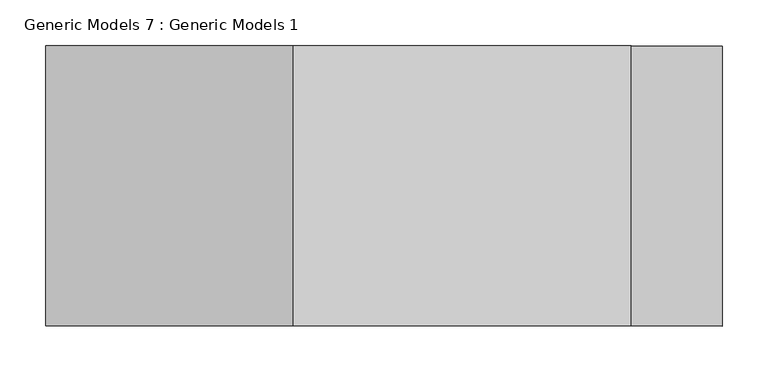
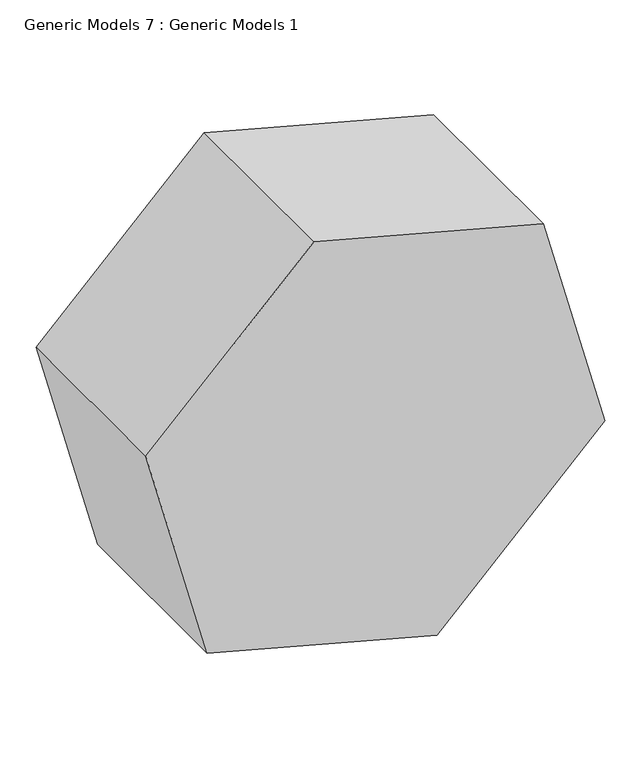
"""IFC4 building model written with IfcOpenShell, lengths in millimetres: proxy geometry, Generic Models 7 : Generic Models 1."""

from ifc_helpers import new_model, si_unit, frame, origin, place, context, project, spatial, polyline, outline, extrude, source, transform, mapped, element, save


def generic_models_7_generic_models_1_35c4f0a6(model_context):
    return source(origin(), model_context, "Body", "SweptSolid", [
        extrude(outline(polyline([(904.7566299, -4463.0070438), (1003.366686, -4831.0247836), (733.9590024, -5100.4324672), (365.9412626, -5001.822411), (267.3312064, -4633.8046712), (536.73889, -4364.3969876), (904.7566299, -4463.0070438)])), frame((0.0, -9086.6225464, 0.0), z_axis=(0.0, 1.0, 0.0), x_axis=(0.0, 0.0, 1.0)), (0.0, 0.0, 1.0), 304.8),
    ])


if __name__ == "__main__":
    model = new_model("IFC4")
    model_context = context("Model", 3, world=origin())
    ifc_project = project(units=[si_unit("LENGTHUNIT", "METRE", prefix="MILLI")], contexts=[model_context])
    site = spatial("IfcSite", under=ifc_project)
    building = spatial("IfcBuilding", under=site)
    placement = place(None, origin())
    generic_models_7_generic_models_1_shape = generic_models_7_generic_models_1_35c4f0a6(model_context)
    element("IfcBuildingElementProxy", 1, Name="Generic Models 7 : Generic Models 1", ObjectType="Generic Models 7 : Generic Models 1", at=placement, inside=building, context=model_context, shape_type="MappedRepresentation", body=[
        mapped(generic_models_7_generic_models_1_shape, transform((0.0, 0.0, 0.0), x_axis=(1.0, 0.0, 0.0), y_axis=(0.0, 1.0, 0.0), z_axis=(0.0, 0.0, 1.0))),
    ])
    save(model, "model.ifc")

# Revit data of these elements
# Element 1 (IfcBuildingElementProxy, "Generic Models 7 : Generic Models 1")
#   Materials on its faces: "Carpet (1)"
# Materials
#   "Carpet (1)": class "Carpet", colour RGB 124 80 67, transparency 0, Description = "Interior finish", Cost = 0
